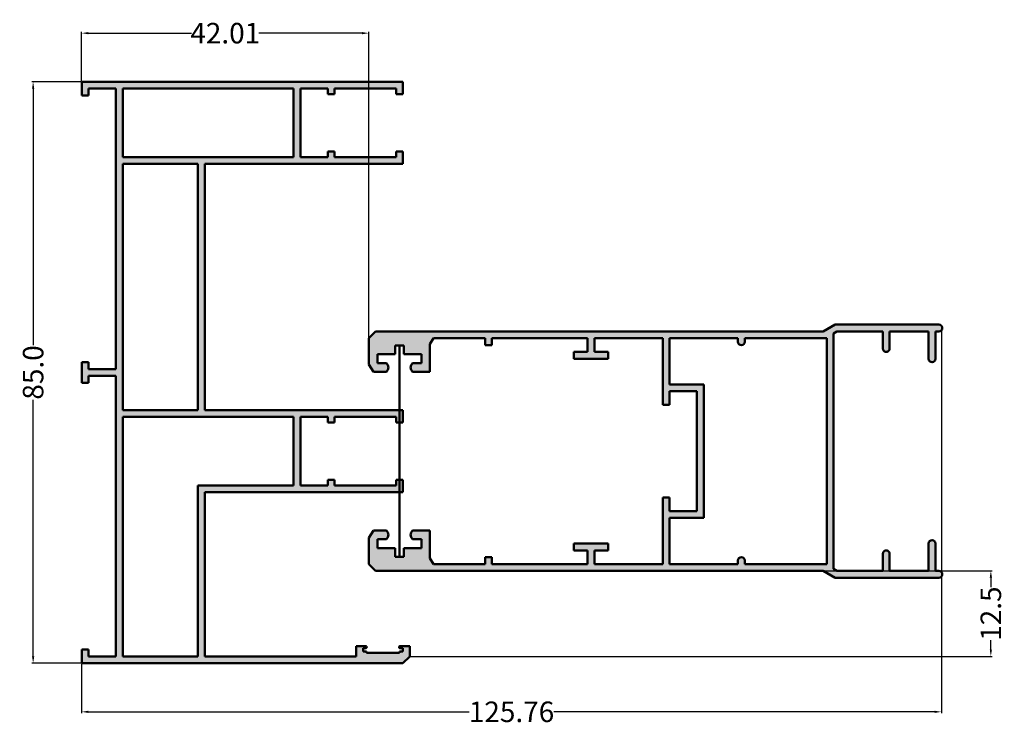
# Model space of a CAD drawing. Units: millimetres. Extents: x 9 to 262, y -226 to 104.
# Tile 1 of 4: x 118 to 262, y -226 to -123. Entities that reach past the tile are written whole.
import ezdxf

# ---------------------------------------------------------------- set-up
doc = ezdxf.new("R2010")
doc.units = ezdxf.units.MM
doc.header["$MEASUREMENT"] = 0
for name, color, linetype, lineweight in [('M-CONS', 8, 'Continuous', 13), ('M-DIMS', 2, 'Continuous', 25), ('M-HATC', 9, 'Continuous', 18), ('M-OUTL', 7, 'Continuous', 50)]:
    doc.layers.add(name, color=color, linetype=linetype, lineweight=lineweight)
doc.styles.get("Standard").update_dxf_attribs({"font": 'arial.ttf'})
doc.dimstyles.get("Standard").update_dxf_attribs({"dimtxt": 3, "dimasz": 1, "dimexe": 0.18, "dimexo": 0.0625, "dimgap": 0.09, "dimtad": 0, "dimdec": 1, "dimzin": 0, "dimdsep": 46, "dimtxsty": 'Standard', "dimcen": 0.09, "dimadec": 0, "dimazin": 0, "dimtfac": 1, "dimtdec": 1, "dimtofl": 0, "dimtmove": 0, "dimatfit": 3, "dimfxl": 1, "dimtolj": 1, "dimtzin": 0, "dimarcsym": 0})

# ---------------------------------------------------------------- blocks, each defined once
blk = doc.blocks.new('PROFILE-FRAME')
for p, q in [((0, 47), (1, 48)), ((1, 48), (2.5, 48)), ((2.5, 48), (2.5, 46.6)), ((0, 47), (0, 0)), ((1.5, 46.5), (1.5, 41.66)), ((1.7, 46.5), (1.5, 46.5)), ((1.7, 47), (2.2, 47)), ((1.7, 47), (2.2, 47)), ((2.2, 47), (1.7, 47)), ((1.7, 47), (1.7, 46.5)), ((2.2, 46.6), (2.2, 47)), ((25, 47), (25, 18)), ((25, 47), (26.8, 47)), ((26.8, 47), (26.8, 46)), ((36, 47), (35.2, 47)), ((35.2, 47), (35.2, 46)), ((35.2, 47), (37, 47)), ((37, 47), (37, 18)), ((73, 47), (73, 18)), ((73, 47), (74.8, 47)), ((74, 47), (74.8, 47)), ((74.8, 47), (74.8, 46)), ((84, 47), (83.2, 47)), ((83.2, 47), (83.2, 46)), ((83.2, 47), (85, 47)), ((85, 47), (85, 0)), ((26, 46), (26, 37)), ((26, 46), (26.8, 46)), ((35.2, 46), (36, 46)), ((35.2, 46), (36, 46)), ((36, 46), (36, 37)), ((74, 46), (74, 37)), ((74, 46), (74.8, 46)), ((83.2, 46), (84, 46)), ((84, 46), (84, 37)), ((1.7, 41.66), (1.5, 41.66)), ((1.7, 41.16), (1.7, 41.66)), ((1.7, 41.16), (2.2, 41.16)), ((1.7, 41.16), (2.2, 41.16)), ((2.2, 41.16), (1.7, 41.16)), ((2.2, 41.56), (2.2, 41.16)), ((2.5, 40.16), (2.5, 41.56)), ((1, 40.16), (2.5, 40.16)), ((1, 40.16), (1, 18)), ((26, 37), (26.8, 37)), ((26.8, 37), (26.8, 36)), ((35.2, 37), (36, 37)), ((35.2, 37), (36, 37)), ((35.2, 37), (35.2, 36)), ((74, 37), (74.8, 37)), ((74.8, 37), (74.8, 36)), ((83.2, 37), (84, 37)), ((83.2, 37), (83.2, 36)), ((26, 36), (26.8, 36)), ((26, 36), (26, 33)), ((35.2, 36), (36, 36)), ((36, 36), (36, 33)), ((74, 36), (74.8, 36)), ((74, 36), (74, 33)), ((83.2, 36), (84, 36)), ((84, 36), (84, 33)), ((26, 33), (26, 32)), ((26, 32), (36, 32)), ((36, 33), (36, 32)), ((74, 33), (74, 32)), ((74, 32), (84, 32)), ((84, 33), (84, 32)), ((26, 31), (36, 31)), ((26, 31), (26, 27)), ((36, 31), (36, 27)), ((74, 31), (84, 31)), ((74, 31), (74, 27)), ((84, 31), (84, 27)), ((26, 27), (26, 17)), ((36, 27), (36, 6)), ((74, 27), (74, 17)), ((84, 27), (84, 17)), ((1, 18), (25, 18)), ((37, 18), (73, 18)), ((1, 17), (26, 17)), ((1, 17), (1, 6)), ((37, 17), (73, 17)), ((37, 17), (37, 6)), ((73, 17), (73, 6)), ((74, 17), (74, 6)), ((84, 17), (84, 6)), ((1, 6), (36, 6)), ((37, 6), (73, 6)), ((74, 6), (84, 6)), ((1, 5), (42, 5)), ((1, 5), (1, 1)), ((42, 5), (42, 1)), ((43, 5), (43, 1)), ((43, 5), (84, 5)), ((84, 5), (84, 1)), ((1, 1), (2, 1)), ((1, 1), (2, 1)), ((2, 1), (2, 0)), ((41, 1), (42, 1)), ((41, 1), (41, 0)), ((43, 1), (44, 1)), ((43, 1), (44, 1)), ((44, 1), (44, 0)), ((84, 1), (83, 1)), ((83, 1), (83, 0)), ((83, 1), (84, 1)), ((0, 0), (2, 0)), ((41, 0), (44, 0)), ((83, 0), (85, 0))]:
    blk.add_line(p, q)
for centre, start, end in [((2.35, 46.6), 180, 0), ((2.35, 41.56), 0, 180)]:
    blk.add_arc(centre, 0.15, start, end)
blk = doc.blocks.new('PROFILE-SASH')
for p, q in [((66.48, 36), (68.21, 37)), ((68.21, 37), (83.4, 37)), ((1, 36), (0, 35)), ((0, 35), (0, 31.15)), ((1, 36), (66.48, 36)), ((8.94, 34.12), (9.45, 35)), ((9.45, 35), (17, 35)), ((17, 35), (17, 34)), ((18, 35), (18, 34)), ((18, 35), (32, 35)), ((32, 35), (32, 33)), ((33, 35), (33, 33)), ((33, 35), (33, 33)), ((33, 35), (43, 35)), ((43, 35), (43, 25.25)), ((44, 35), (44, 28.25)), ((44, 35), (54, 35)), ((54, 35), (54, 34.5)), ((55, 35), (55, 34.5)), ((55, 35), (67, 35)), ((55, 35), (66.48, 35)), ((67, 35), (67, 2)), ((68, 35.72), (68.48, 36)), ((68, 35.72), (68, 1.28)), ((68.48, 36), (75.19, 36)), ((75.19, 36), (75.19, 33.5)), ((76.19, 36), (76.19, 33.5)), ((76.19, 36), (81.9, 36)), ((81.9, 36), (81.9, 32)), ((82.9, 36), (82.9, 32)), ((82.9, 36), (83.4, 36)), ((3.85, 32.67), (3.85, 33.95)), ((3.85, 33.95), (5.13, 33.95)), ((5.13, 32.67), (5.13, 33.95)), ((8.94, 30.1), (8.94, 34.12)), ((17, 34), (18, 34)), ((1.28, 31.38), (1.28, 32.67)), ((1.28, 31.38), (1.28, 32.67)), ((1.28, 32.67), (3.85, 32.67)), ((7.7, 32.67), (5.13, 32.67)), ((7.7, 31.38), (7.7, 32.67)), ((30, 32), (30, 33)), ((30, 33), (32, 33)), ((32, 32), (30, 32)), ((35, 32), (32, 32)), ((33, 33), (35, 33)), ((35, 33), (35, 32)), ((0, 31.15), (0.69, 30.1)), ((2.61, 31.38), (1.28, 31.38)), ((6.37, 31.38), (7.7, 31.38)), ((0.69, 30.1), (2.61, 30.1)), ((6.37, 30.1), (8.94, 30.1)), ((44, 28.25), (49, 28.25)), ((49, 28.25), (49, 8.75)), ((44, 27.25), (48, 27.25)), ((44, 27.25), (44, 25.25)), ((48, 27.25), (48, 9.75)), ((43, 25.25), (44, 25.25)), ((43, 11.75), (44, 11.75)), ((43, 11.75), (43, 2)), ((44, 11.75), (44, 9.75)), ((48, 9.75), (44, 9.75)), ((49, 8.75), (44, 8.75)), ((44, 8.75), (44, 2)), ((0, 5.85), (0.69, 6.9)), ((0, 5.85), (0, 2)), ((0.69, 6.9), (2.61, 6.9)), ((6.37, 6.9), (8.94, 6.9)), ((8.94, 6.9), (8.94, 2.88)), ((1.28, 5.62), (1.28, 4.33)), ((2.61, 5.62), (1.28, 5.62)), ((1.28, 5.62), (1.28, 4.33)), ((1.28, 4.33), (3.85, 4.33)), ((3.85, 4.33), (3.85, 3.05)), ((7.7, 4.33), (5.13, 4.33)), ((5.13, 4.33), (5.13, 3.05)), ((6.37, 5.62), (7.7, 5.62)), ((7.7, 5.62), (7.7, 4.33)), ((32, 5), (30, 5)), ((30, 5), (30, 4)), ((35, 5), (32, 5)), ((35, 4), (35, 5)), ((81.9, 5), (81.9, 1)), ((82.9, 5), (82.9, 1)), ((3.85, 3.05), (5.13, 3.05)), ((17, 3), (18, 3)), ((17, 3), (17, 2)), ((18, 3), (18, 2)), ((30, 4), (32, 4)), ((32, 4), (32, 2)), ((33, 2), (33, 4)), ((33, 4), (35, 4)), ((33, 4), (33, 2)), ((75.19, 3.5), (75.19, 1)), ((76.19, 3.5), (76.19, 1)), ((0, 2), (1, 1)), ((8.94, 2.88), (9.45, 2)), ((9.45, 2), (17, 2)), ((18, 2), (32, 2)), ((33, 2), (43, 2)), ((44, 2), (54, 2)), ((44, 2), (54, 2)), ((54, 2.5), (54, 2)), ((55, 2.5), (55, 2)), ((55, 2), (67, 2)), ((55, 2), (66.48, 2)), ((1, 1), (66.48, 1)), ((66.48, 1), (68.21, 0)), ((68, 1.28), (68.48, 1)), ((68.48, 1), (75.19, 1)), ((76.19, 1), (81.9, 1)), ((76.19, 1), (81.9, 1)), ((82.9, 1), (83.4, 1)), ((82.9, 1), (83.4, 1)), ((68.21, 0), (83.4, 0))]:
    blk.add_line(p, q)
for centre, radius, start, end in [((83.4, 36.5), 0.5, 270, 90), ((54.5, 34.5), 0.5, 180, 0), ((75.69, 33.5), 0.5, 180, 0), ((82.4, 32), 0.5, 180, 0), ((1.96, 30.74), 0.911, 315.2177, 44.7823), ((7.02, 30.74), 0.911, 135.2177, 224.7823), ((1.96, 6.26), 0.911, 315.2177, 44.7823), ((7.02, 6.26), 0.911, 135.2177, 224.7823), ((82.4, 5), 0.5, 0, 180), ((54.5, 2.5), 0.5, 0, 180), ((75.69, 3.5), 0.5, 0, 180), ((83.4, 0.5), 0.5, 270, 90)]:
    blk.add_arc(centre, radius, start, end)
blk = doc.blocks.new('*D31')
at = {"layer": 'Defpoints', "color": 0, "transparency": 16777216}
for p in [(252.6, -167.75), (126.83, -217.1), (252.6, -224.2)]:
    blk.add_point(p, dxfattribs=at)
at = {"layer": 'M-DIMS', "color": 0, "lineweight": -2, "transparency": 16777216}
for p, q in [((252.6, -167.81), (252.6, -224.38)), ((126.83, -217.17), (126.83, -224.38)), ((127.83, -224.2), (183.54, -224.2)), ((251.6, -224.2), (195.89, -224.2))]:
    blk.add_line(p, q, dxfattribs=at)
at = {"layer": 'M-DIMS', "color": 0, "transparency": 16777216}
for points in [[(127.83, -224.04), (127.83, -224.37), (126.83, -224.2)], [(251.6, -224.04), (251.6, -224.37), (252.6, -224.2)]]:
    blk.add_solid(points, dxfattribs=at)
at = {"layer": 'M-DIMS', "color": 0, "transparency": 16777216, "insert": (189.72, -224.2), "char_height": 3, "attachment_point": 5}
blk.add_mtext('\\A1;125.76', dxfattribs=at)
blk = doc.blocks.new('*D32')
at = {"layer": 'Defpoints', "color": 0, "transparency": 16777216}
for p in [(168.84, -125), (126.83, -132.1), (168.84, -173.45)]:
    blk.add_point(p, dxfattribs=at)
at = {"layer": 'M-DIMS', "color": 0, "lineweight": -2, "transparency": 16777216}
for p, q in [((126.83, -132.04), (126.83, -124.82)), ((127.83, -125), (142.92, -125)), ((167.84, -125), (152.76, -125)), ((168.84, -173.39), (168.84, -124.82))]:
    blk.add_line(p, q, dxfattribs=at)
at = {"layer": 'M-DIMS', "color": 0, "transparency": 16777216}
for points in [[(127.83, -124.84), (127.83, -125.17), (126.83, -125)], [(167.84, -124.84), (167.84, -125.17), (168.84, -125)]]:
    blk.add_solid(points, dxfattribs=at)
at = {"layer": 'M-DIMS', "color": 0, "transparency": 16777216, "insert": (147.84, -125), "char_height": 3, "attachment_point": 5}
blk.add_mtext('\\A1;42.01', dxfattribs=at)
blk = doc.blocks.new('*D33')
at = {"layer": 'Defpoints', "color": 0, "transparency": 16777216}
for p in [(119.73, -132.1), (126.83, -132.1), (126.83, -217.1)]:
    blk.add_point(p, dxfattribs=at)
at = {"layer": 'M-DIMS', "color": 0, "lineweight": -2, "transparency": 16777216}
for p, q in [((126.77, -132.1), (119.55, -132.1)), ((119.73, -133.1), (119.73, -170.62)), ((119.73, -216.1), (119.73, -178.59)), ((126.77, -217.1), (119.55, -217.1))]:
    blk.add_line(p, q, dxfattribs=at)
at = {"layer": 'M-DIMS', "color": 0, "transparency": 16777216}
for points in [[(119.57, -133.1), (119.9, -133.1), (119.73, -132.1)], [(119.57, -216.1), (119.9, -216.1), (119.73, -217.1)]]:
    blk.add_solid(points, dxfattribs=at)
at = {"layer": 'M-DIMS', "color": 0, "transparency": 16777216, "insert": (119.73, -174.6), "char_height": 3, "attachment_point": 5, "rotation": 90}
blk.add_mtext('\\A1;85.0', dxfattribs=at)
blk = doc.blocks.new('*D34')
at = {"layer": 'Defpoints', "color": 0, "transparency": 16777216}
for p in [(169.84, -203.6), (174.83, -216.1), (259.84, -216.1)]:
    blk.add_point(p, dxfattribs=at)
at = {"layer": 'M-DIMS', "color": 0, "lineweight": -2, "transparency": 16777216}
for p, q in [((169.91, -203.6), (260.02, -203.6)), ((259.84, -204.6), (259.84, -206)), ((259.84, -215.1), (259.84, -213.71)), ((174.9, -216.1), (260.02, -216.1))]:
    blk.add_line(p, q, dxfattribs=at)
at = {"layer": 'M-DIMS', "color": 0, "transparency": 16777216}
for points in [[(259.68, -204.6), (260.01, -204.6), (259.84, -203.6)], [(259.68, -215.1), (260.01, -215.1), (259.84, -216.1)]]:
    blk.add_solid(points, dxfattribs=at)
at = {"layer": 'M-DIMS', "color": 0, "transparency": 16777216, "insert": (259.84, -209.85), "char_height": 3, "attachment_point": 5, "rotation": 90}
blk.add_mtext('\\A1;12.5', dxfattribs=at)

msp = doc.modelspace()

# ---------------------------------------------------------------- hatches: boundary and pattern name
at = {"layer": 'M-HATC'}
h = msp.add_hatch(color=256, dxfattribs=at)
h.dxf.hatch_style = 1
h.paths.add_polyline_path([(173.8347, -180.1039), (173.8347, -181.9039), (172.8347, -181.9039), (172.8347, -181.1039), (163.8347, -181.1039), (163.8347, -181.9039), (162.8347, -181.9039), (162.8347, -181.1039), (159.8347, -181.1039), (158.8347, -181.1039), (158.8347, -191.1039), (159.8347, -191.1039), (162.8347, -191.1039), (162.8347, -190.3039), (163.8347, -190.3039), (163.8347, -191.1039), (172.8347, -191.1039), (172.8347, -190.3039), (173.8347, -190.3039), (173.8347, -192.1039), (144.8347, -192.1039), (144.8347, -216.1039), (166.9938, -216.1039), (166.9938, -214.6039), (168.3938, -214.6039, -1), (168.3938, -214.9039), (167.9938, -214.9039), (167.9938, -215.4039), (168.4938, -215.4039), (168.4938, -215.6039), (173.3347, -215.6039), (173.3347, -215.4039), (173.8347, -215.4039), (173.8347, -214.9039), (173.4347, -214.9039, -1), (173.4347, -214.6039), (174.8347, -214.6039), (174.8347, -216.1039), (173.8347, -217.1039), (126.8347, -217.1039), (126.8347, -215.1039), (127.8347, -215.1039), (127.8347, -216.1039), (131.8347, -216.1039), (131.8347, -175.1039), (127.8347, -175.1039), (127.8347, -176.1039), (126.8347, -176.1039), (126.8347, -173.1039), (127.8347, -173.1039), (127.8347, -174.1039), (131.8347, -174.1039), (131.8347, -133.1039), (127.8347, -133.1039), (127.8347, -134.1039), (126.8347, -134.1039), (126.8347, -132.1039), (173.8347, -132.1039), (173.8347, -133.9039), (172.8347, -133.9039), (172.8347, -133.1039), (163.8347, -133.1039), (163.8347, -133.9039), (162.8347, -133.9039), (162.8347, -133.1039), (159.8347, -133.1039), (158.8347, -133.1039), (158.8347, -143.1039), (159.8347, -143.1039), (162.8347, -143.1039), (162.8347, -142.3039), (163.8347, -142.3039), (163.8347, -143.1039), (172.8347, -143.1039), (172.8347, -142.3039), (173.8347, -142.3039), (173.8347, -143.1039), (173.8347, -144.1039), (144.8347, -144.1039), (144.8347, -180.1039)])
h.paths.add_polyline_path([(157.8347, -181.1039), (153.8347, -181.1039), (132.8347, -181.1039), (132.8347, -216.1039), (143.8347, -216.1039), (143.8347, -191.1039), (153.8347, -191.1039), (157.8347, -191.1039)], flags=16)
h.paths.add_polyline_path([(143.8347, -180.1039), (143.8347, -144.1039), (132.8347, -144.1039), (132.8347, -180.1039)], flags=16)
h.paths.add_polyline_path([(157.8347, -143.1039), (157.8347, -133.1039), (153.8347, -133.1039), (143.8347, -133.1039), (132.8347, -133.1039), (132.8347, -143.1039), (143.8347, -143.1039), (153.8347, -143.1039)], flags=16)
h = msp.add_hatch(color=256, dxfattribs=at)
h.dxf.hatch_style = 1
h.paths.add_polyline_path([(211.8427, -202.6039), (201.8427, -202.6039), (201.8427, -200.6039), (203.8427, -200.6039), (203.8427, -199.6039), (200.8427, -199.6039), (198.8427, -199.6039), (198.8427, -200.6039), (200.8427, -200.6039), (200.8427, -202.6039), (186.8427, -202.6039), (186.8427, -201.6039), (185.8427, -201.6039), (185.8427, -202.6039), (178.2915, -202.6039), (177.7837, -201.7244), (177.7837, -197.7049), (175.2168, -197.7049, 0.4119899), (175.2168, -198.9883), (176.5434, -198.9883), (176.5434, -200.2718), (173.9765, -200.2718), (173.9765, -201.5552), (172.693, -201.5552), (172.693, -200.2718), (170.1261, -200.2718), (170.1261, -198.9883), (171.4527, -198.9883, 0.4119899), (171.4527, -197.7049), (169.5276, -197.7049), (168.8427, -198.7535), (168.8427, -202.6039), (169.8427, -203.6039), (235.3196, -203.6039), (237.0517, -204.6039), (252.2427, -204.6039, 1), (252.2427, -203.6039), (251.7427, -203.6039), (251.7427, -199.6039, 1), (250.7427, -199.6039), (250.7427, -203.6039), (245.0311, -203.6039), (245.0311, -201.1039, 1), (244.0311, -201.1039), (244.0311, -203.6039), (237.3196, -203.6039), (236.8427, -203.3285), (236.8427, -168.8793), (237.3196, -168.6039), (244.0311, -168.6039), (244.0311, -171.1039, 1), (245.0311, -171.1039), (245.0311, -168.6039), (250.7427, -168.6039), (250.7427, -172.6039, 1), (251.7427, -172.6039), (251.7427, -168.6039), (252.2427, -168.6039, 1), (252.2427, -167.6039), (237.0517, -167.6039), (235.3196, -168.6039), (169.8427, -168.6039), (168.8427, -169.6039), (168.8427, -173.4543), (169.5276, -174.5029), (171.4527, -174.5029, 0.4119899), (171.4527, -173.2195), (170.1261, -173.2195), (170.1261, -171.936), (172.693, -171.936), (172.693, -170.6526), (173.9765, -170.6526), (173.9765, -171.936), (176.5434, -171.936), (176.5434, -173.2195), (175.2168, -173.2195, 0.4119899), (175.2168, -174.5029), (177.7837, -174.5029), (177.7837, -170.4834), (178.2915, -169.6039), (185.8427, -169.6039), (185.8427, -170.6039), (186.8427, -170.6039), (186.8427, -169.6039), (200.8427, -169.6039), (200.8427, -171.6039), (198.8427, -171.6039), (198.8427, -172.6039), (200.8427, -172.6039), (203.8427, -172.6039), (203.8427, -171.6039), (201.8427, -171.6039), (201.8427, -169.6039), (211.8427, -169.6039), (211.8427, -179.3539), (212.8427, -179.3539), (212.8427, -177.3539), (216.8427, -177.3539), (216.8427, -194.8539), (212.8427, -194.8539), (212.8427, -192.8539), (211.8427, -192.8539)])
h.paths.add_polyline_path([(212.8427, -195.8539), (217.8427, -195.8539), (217.8427, -176.3539), (212.8427, -176.3539), (212.8427, -169.6039), (222.8427, -169.6039), (222.8427, -170.1039, 1), (223.8427, -170.1039), (223.8427, -169.6039), (235.8427, -169.6039), (235.8427, -202.6039), (223.8427, -202.6039), (223.8427, -202.1039, 1), (222.8427, -202.1039), (222.8427, -202.6039), (212.8427, -202.6039)], flags=16)

# ---------------------------------------------------------------- linework, layer by layer
at = {"layer": 'M-CONS'}
for p in [(211.8427, -177.3539), (211.8427, -194.8539)]:
    msp.add_point(p, dxfattribs=at)
at = {"layer": 'M-OUTL'}
for p, q in [((173.3347, -170.6526), (173.3347, -201.5552)), ((173.3347, -181.9039), (173.3347, -190.3039))]:
    msp.add_line(p, q, dxfattribs=at)

# ---------------------------------------------------------------- block references
at = {"layer": 'M-OUTL', "extrusion": (0, 0, -1), "zscale": -1, "rotation": 90.00000000000048}
msp.add_blockref('PROFILE-FRAME', (-126.8348, -217.1041), dxfattribs=at)
at = {"layer": 'M-OUTL'}
msp.add_blockref('PROFILE-SASH', (168.8423, -204.6038), dxfattribs=at)

# ---------------------------------------------------------------- dimensions: what is measured, and where the dimension line sits
at = {"layer": 'M-DIMS'}
for base, p1, p2, picture, middle in [((168.8427, -125.0039), (126.8347, -132.1039), (168.8427, -173.4543), '*D32', (147.8387, -125.0039)), ((252.5962, -224.2039), (126.8347, -217.1039), (252.5962, -167.7503), '*D31', (189.7155, -224.2039))]:
    dim = msp.add_linear_dim(base=base, p1=p1, p2=p2, dimstyle='Standard', override={"dimdec": 2, "dimlfac": 1, "dimrnd": 0, "dimzin": 0, "dimdsep": 46, "dimlunit": 2}, dxfattribs=at)
    dim.commit()
    dim.dimension.update_dxf_attribs({"geometry": picture, "text_midpoint": middle})
for base, p1, p2, picture, middle in [((119.7347, -132.1039), (126.8347, -217.1039), (126.8347, -132.1039), '*D33', (119.7347, -174.6039)), ((259.8427, -216.1039), (169.8427, -203.6039), (174.8347, -216.1039), '*D34', (259.8427, -209.8539))]:
    dim = msp.add_linear_dim(base=base, p1=p1, p2=p2, angle=90, dimstyle='Standard', override={"dimdec": 1, "dimlfac": 1, "dimrnd": 0, "dimzin": 0, "dimdsep": 46, "dimlunit": 2}, dxfattribs=at)
    dim.commit()
    dim.dimension.update_dxf_attribs({"geometry": picture, "text_midpoint": middle})

doc.saveas('drawing.dxf')
